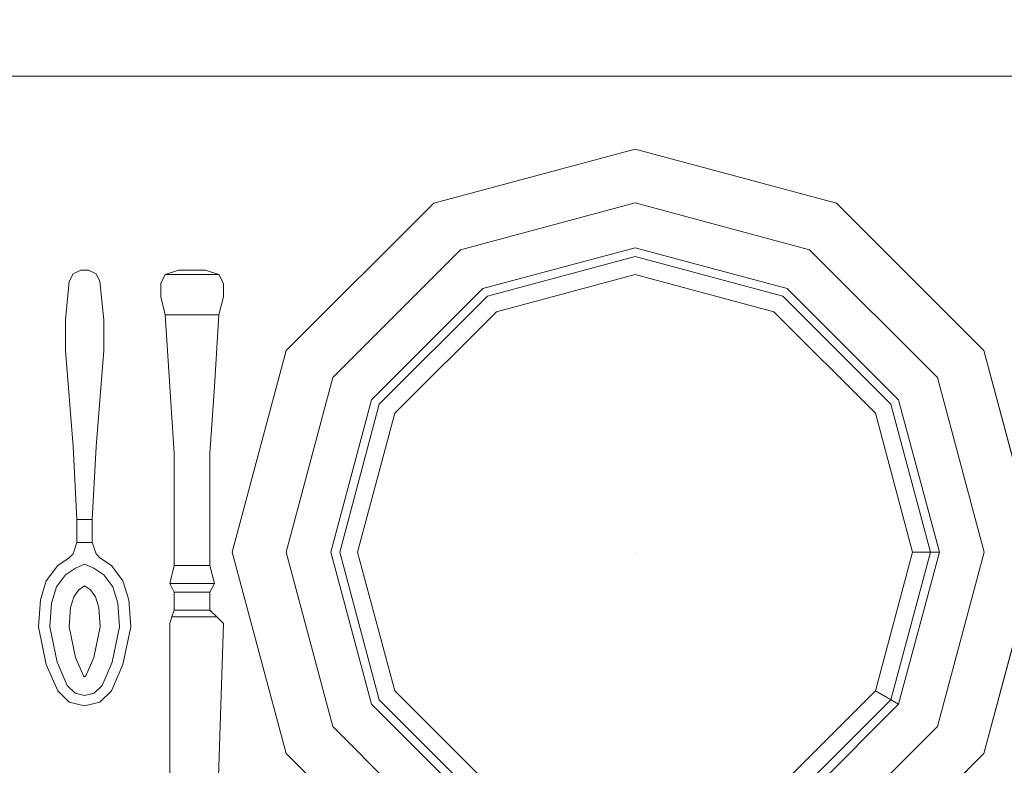
# Model space of a CAD drawing. Units: inches. Extents: x 375 to 1122, y 27 to 1069.
# Tile 135 of 155: x 717.62 to 731.16, y 906.27 to 916.52. Entities that reach past the tile are written whole.
import ezdxf

# ---------------------------------------------------------------- set-up
doc = ezdxf.new("R2010")
doc.units = ezdxf.units.IN
doc.layers.add('A-ANNO-DIMS', color=2, linetype='Continuous', lineweight=18)
doc.layers.add('Furniture', color=30, linetype='Continuous', lineweight=18)
doc.styles.get("Standard").update_dxf_attribs({"font": 'arial.ttf'})
doc.dimstyles.new('ISO-25', dxfattribs={"dimtxt": 12, "dimasz": 2.5, "dimexe": 1.5, "dimexo": 1.5, "dimtad": 1, "dimdec": 1, "dimlunit": 3, "dimtxsty": 'Standard', "dimblk": 'ARCHTICK', "dimcen": 2.5, "dimadec": 0, "dimazin": 0, "dimtfac": 1, "dimtdec": 1, "dimtmove": 0, "dimatfit": 3, "dimfxl": 1.5, "dimfxlon": 1, "dimarcsym": 0})

# ---------------------------------------------------------------- blocks, each defined once
blk = doc.blocks.new('A$C403C54AD')
blk.add_line((0.56427, 0.79569, -0.0006), (0.56427, 1.26108, -0.0006))
at = {"linetype": 'ByBlock'}
for points, invisible_edges in [([(0.72796, 1.16691, -0.0197), (0.72796, 1.14844, -0.0197), (0.66793, 1.13235, -0.0197), (0.6587, 1.14835, -0.0197)], 5), ([(0.72796, 1.13305, -0.03355), (0.72796, 1.16691, -0.02431), (0.6587, 1.14835, -0.02431), (0.67563, 1.11902, -0.03355)], 5), ([(0.79723, 1.14835, -0.0197), (0.78799, 1.13235, -0.0197), (0.72796, 1.14844, -0.0197), (0.72796, 1.16691, -0.0197)], 5), ([(0.7803, 1.11902, -0.03355), (0.79723, 1.14835, -0.02431), (0.72796, 1.16691, -0.02431), (0.72796, 1.13305, -0.03355)], 5), ([(0.6587, 1.14835, -0.0197), (0.66793, 1.13235, -0.0197), (0.62399, 1.08841, -0.0197), (0.60799, 1.09765, -0.0197)], 5), ([(0.67563, 1.11902, -0.03355), (0.6587, 1.14835, -0.02431), (0.60799, 1.09765, -0.02431), (0.63732, 1.08071, -0.03355)], 5), ([(0.72796, 1.14844, -0.0197), (0.72796, 1.12997, -0.02585), (0.67717, 1.11636, -0.02585), (0.66793, 1.13235, -0.0197)], 5), ([(0.78799, 1.13235, -0.0197), (0.77876, 1.11636, -0.02585), (0.72796, 1.12997, -0.02585), (0.72796, 1.14844, -0.0197)], 5), ([(0.81861, 1.08071, -0.03355), (0.84793, 1.09765, -0.02431), (0.79723, 1.14835, -0.02431), (0.7803, 1.11902, -0.03355)], 5), ([(0.84793, 1.09765, -0.0197), (0.83194, 1.08841, -0.0197), (0.78799, 1.13235, -0.0197), (0.79723, 1.14835, -0.0197)], 5), ([(0.66793, 1.13235, -0.0197), (0.67717, 1.11636, -0.02585), (0.63999, 1.07918, -0.02585), (0.62399, 1.08841, -0.0197)], 5), ([(0.72796, 1.12381, -0.04278), (0.72796, 1.13305, -0.03355), (0.67563, 1.11902, -0.03355), (0.68025, 1.11103, -0.04278)], 4), ([(0.83194, 1.08841, -0.0197), (0.81594, 1.07918, -0.02585), (0.77876, 1.11636, -0.02585), (0.78799, 1.13235, -0.0197)], 5), ([(0.72796, 1.12997, -0.02585), (0.72796, 1.02838, -0.02585), (0.72796, 1.02838, -0.02585), (0.67717, 1.11636, -0.02585)], 5), ([(0.77876, 1.11636, -0.02585), (0.72796, 1.02838, -0.02585), (0.72796, 1.02838, -0.02585), (0.72796, 1.12997, -0.02585)], 5), ([(0.68025, 1.11103, -0.04278), (0.67563, 1.11902, -0.03355), (0.63732, 1.08071, -0.03355), (0.64532, 1.0761, -0.04278)], 5), ([(0.81061, 1.0761, -0.04278), (0.81861, 1.08071, -0.03355), (0.7803, 1.11902, -0.03355), (0.77568, 1.11103, -0.04278)], 1), ([(0.67717, 1.11636, -0.02585), (0.72796, 1.02838, -0.02585), (0.72796, 1.02838, -0.02585), (0.63999, 1.07918, -0.02585)], 5), ([(0.81594, 1.07918, -0.02585), (0.72796, 1.02838, -0.02585), (0.72796, 1.02838, -0.02585), (0.77876, 1.11636, -0.02585)], 5), ([(0.60799, 1.09765, -0.0197), (0.62399, 1.08841, -0.0197), (0.60791, 1.02838, -0.0197), (0.58944, 1.02838, -0.0197)], 5), ([(0.63732, 1.08071, -0.03355), (0.60799, 1.09765, -0.02431), (0.58944, 1.02838, -0.02431), (0.6233, 1.02838, -0.03355)], 5), ([(0.62399, 1.08841, -0.0197), (0.63999, 1.07918, -0.02585), (0.62638, 1.02838, -0.02585), (0.60791, 1.02838, -0.0197)], 5), ([(0.64532, 1.0761, -0.04278), (0.63732, 1.08071, -0.03355), (0.6233, 1.02838, -0.03355), (0.63253, 1.02838, -0.04278)], 5), ([(0.63999, 1.07918, -0.02585), (0.72796, 1.02838, -0.02585), (0.72796, 1.02838, -0.02585), (0.62638, 1.02838, -0.02585)], 5), ([(0.82955, 1.02838, -0.02585), (0.72796, 1.02838, -0.02585), (0.72796, 1.02838, -0.02585), (0.81594, 1.07918, -0.02585)], 5), ([(0.58944, 1.02838, -0.0197), (0.60791, 1.02838, -0.0197), (0.62399, 0.96835, -0.0197), (0.60799, 0.95912, -0.0197)], 5), ([(0.6233, 1.02838, -0.03355), (0.58944, 1.02838, -0.02431), (0.60799, 0.95912, -0.02431), (0.63732, 0.97605, -0.03355)], 5), ([(0.60791, 1.02838, -0.0197), (0.62638, 1.02838, -0.02585), (0.63999, 0.97759, -0.02585), (0.62399, 0.96835, -0.0197)], 5), ([(0.63253, 1.02838, -0.04278), (0.6233, 1.02838, -0.03355), (0.63732, 0.97605, -0.03355), (0.64532, 0.98067, -0.04278)], 5), ([(0.62638, 1.02838, -0.02585), (0.72796, 1.02838, -0.02585), (0.72796, 1.02838, -0.02585), (0.63999, 0.97759, -0.02585)], 5), ([(0.63999, 0.97759, -0.02585), (0.72796, 1.02838, -0.02585), (0.72796, 1.02838, -0.02585), (0.67717, 0.94041, -0.02585)], 5), ([(0.67717, 0.94041, -0.02585), (0.72796, 1.02838, -0.02585), (0.72796, 1.02838, -0.02585), (0.72796, 0.9268, -0.02585)], 5), ([(0.81594, 0.97759, -0.02585), (0.72796, 1.02838, -0.02585), (0.72796, 1.02838, -0.02585), (0.82955, 1.02838, -0.02585)], 5), ([(0.77876, 0.94041, -0.02585), (0.72796, 1.02838, -0.02585), (0.72796, 1.02838, -0.02585), (0.81594, 0.97759, -0.02585)], 5), ([(0.72796, 0.9268, -0.02585), (0.72796, 1.02838, -0.02585), (0.72796, 1.02838, -0.02585), (0.77876, 0.94041, -0.02585)], 5), ([(0.64532, 0.98067, -0.04278), (0.63732, 0.97605, -0.03355), (0.67563, 0.93774, -0.03355), (0.68025, 0.94574, -0.04278)], 5), ([(0.77568, 0.94574, -0.04278), (0.7803, 0.93774, -0.03355), (0.81861, 0.97605, -0.03355), (0.81061, 0.98067, -0.04278)], 5), ([(0.63732, 0.97605, -0.03355), (0.60799, 0.95912, -0.02431), (0.6587, 0.90841, -0.02431), (0.67563, 0.93774, -0.03355)], 5), ([(0.62399, 0.96835, -0.0197), (0.63999, 0.97759, -0.02585), (0.67717, 0.94041, -0.02585), (0.66793, 0.92441, -0.0197)], 5), ([(0.78799, 0.92441, -0.0197), (0.77876, 0.94041, -0.02585), (0.81594, 0.97759, -0.02585), (0.83194, 0.96835, -0.0197)], 5), ([(0.7803, 0.93774, -0.03355), (0.79723, 0.90841, -0.02431), (0.84793, 0.95912, -0.02431), (0.81861, 0.97605, -0.03355)], 5), ([(0.60799, 0.95912, -0.0197), (0.62399, 0.96835, -0.0197), (0.66793, 0.92441, -0.0197), (0.6587, 0.90841, -0.0197)], 5), ([(0.79723, 0.90841, -0.0197), (0.78799, 0.92441, -0.0197), (0.83194, 0.96835, -0.0197), (0.84793, 0.95912, -0.0197)], 5), ([(0.68025, 0.94574, -0.04278), (0.67563, 0.93774, -0.03355), (0.72796, 0.92372, -0.03355), (0.72796, 0.93295, -0.04278)], 5), ([(0.72796, 0.93295, -0.04278), (0.72796, 0.92372, -0.03355), (0.7803, 0.93774, -0.03355), (0.77568, 0.94574, -0.04278)], 5), ([(0.66793, 0.92441, -0.0197), (0.67717, 0.94041, -0.02585), (0.72796, 0.9268, -0.02585), (0.72796, 0.90833, -0.0197)], 5), ([(0.72796, 0.90833, -0.0197), (0.72796, 0.9268, -0.02585), (0.77876, 0.94041, -0.02585), (0.78799, 0.92441, -0.0197)], 5), ([(0.67563, 0.93774, -0.03355), (0.6587, 0.90841, -0.02431), (0.72796, 0.88985, -0.02431), (0.72796, 0.92372, -0.03355)], 5), ([(0.72796, 0.92372, -0.03355), (0.72796, 0.88985, -0.02431), (0.79723, 0.90841, -0.02431), (0.7803, 0.93774, -0.03355)], 5), ([(0.6587, 0.90841, -0.0197), (0.66793, 0.92441, -0.0197), (0.72796, 0.90833, -0.0197), (0.72796, 0.88985, -0.0197)], 5), ([(0.72796, 0.88985, -0.0197), (0.72796, 0.90833, -0.0197), (0.78799, 0.92441, -0.0197), (0.79723, 0.90841, -0.0197)], 5)]:
    blk.add_3dface(points, dxfattribs=dict(at, invisible_edges=invisible_edges))
for points in [[(0.72796, 1.16691, -0.02431), (0.72796, 1.16691, -0.0197), (0.6587, 1.14835, -0.0197), (0.6587, 1.14835, -0.02431)], [(0.79723, 1.14835, -0.02431), (0.79723, 1.14835, -0.0197), (0.72796, 1.16691, -0.0197), (0.72796, 1.16691, -0.02431)], [(0.6587, 1.14835, -0.02431), (0.6587, 1.14835, -0.0197), (0.60799, 1.09765, -0.0197), (0.60799, 1.09765, -0.02431)], [(0.84793, 1.09765, -0.02431), (0.84793, 1.09765, -0.0197), (0.79723, 1.14835, -0.0197), (0.79723, 1.14835, -0.02431)], [(0.77568, 1.11103, -0.04278), (0.7803, 1.11902, -0.03355), (0.72796, 1.13305, -0.03355), (0.72796, 1.12381, -0.04278)], [(0.60799, 1.09765, -0.02431), (0.60799, 1.09765, -0.0197), (0.58944, 1.02838, -0.0197), (0.58944, 1.02838, -0.02431)], [(0.58944, 1.02838, -0.02431), (0.58944, 1.02838, -0.0197), (0.60799, 0.95912, -0.0197), (0.60799, 0.95912, -0.02431)], [(0.60799, 0.95912, -0.02431), (0.60799, 0.95912, -0.0197), (0.6587, 0.90841, -0.0197), (0.6587, 0.90841, -0.02431)], [(0.79723, 0.90841, -0.02431), (0.79723, 0.90841, -0.0197), (0.84793, 0.95912, -0.0197), (0.84793, 0.95912, -0.02431)], [(0.6587, 0.90841, -0.02431), (0.6587, 0.90841, -0.0197), (0.72796, 0.88985, -0.0197), (0.72796, 0.88985, -0.02431)], [(0.72796, 0.88985, -0.02431), (0.72796, 0.88985, -0.0197), (0.79723, 0.90841, -0.0197), (0.79723, 0.90841, -0.02431)]]:
    blk.add_3dface(points, dxfattribs=at)
for points in [[(0.63253, 0.88524, -0.03355), (0.63253, 0.86677, -0.03355), (0.63099, 0.87138, -0.03663), (0.63099, 0.88062, -0.03663)], [(0.63253, 0.88524, -0.03355), (0.63253, 0.88524, -0.03971), (0.63099, 0.88062, -0.03663)], [(0.63253, 0.88524, -0.03971), (0.63253, 0.86677, -0.03971), (0.63099, 0.87138, -0.03663), (0.63099, 0.88062, -0.03663)], [(0.63561, 0.88678, -0.04124), (0.63561, 0.88678, -0.03201), (0.63253, 0.88524, -0.03355), (0.63253, 0.88524, -0.03971)], [(0.64023, 0.88678, -0.03047), (0.64023, 0.88678, -0.04278), (0.63561, 0.88678, -0.04124), (0.63561, 0.88678, -0.03201)], [(0.64639, 0.88524, -0.04124), (0.64639, 0.88524, -0.03201), (0.64023, 0.88678, -0.03047), (0.64023, 0.88678, -0.04278)], [(0.67101, 0.8837, -0.03047), (0.67101, 0.8837, -0.04278), (0.64639, 0.88524, -0.04124), (0.64639, 0.88524, -0.03201)], [(0.75028, 0.88447, -0.03509), (0.75028, 0.86908, -0.03509), (0.74797, 0.86985, -0.03201), (0.74797, 0.88216, -0.03201)], [(0.75028, 0.88447, -0.03817), (0.75028, 0.86908, -0.03817), (0.74797, 0.86985, -0.04124), (0.74797, 0.88216, -0.04124)], [(0.6941, 0.88216, -0.04278), (0.6941, 0.88216, -0.03047), (0.67101, 0.8837, -0.03047), (0.67101, 0.8837, -0.04278)], [(0.73258, 0.88216, -0.03201), (0.73258, 0.88216, -0.04124), (0.6941, 0.88216, -0.04278), (0.6941, 0.88216, -0.03047)], [(0.73874, 0.86831, -0.03047), (0.73874, 0.8837, -0.03047), (0.73258, 0.88216, -0.03201), (0.73258, 0.86985, -0.03201)], [(0.73874, 0.86831, -0.04278), (0.73874, 0.8837, -0.04278), (0.73258, 0.88216, -0.04124), (0.73258, 0.86985, -0.04124)], [(0.73874, 0.8837, -0.04278), (0.73874, 0.8837, -0.03047), (0.73258, 0.88216, -0.03201), (0.73258, 0.88216, -0.04124)], [(0.74182, 0.88216, -0.03201), (0.74182, 0.86985, -0.03201), (0.73874, 0.86831, -0.03047), (0.73874, 0.8837, -0.03047)], [(0.74182, 0.88216, -0.04124), (0.74182, 0.86985, -0.04124), (0.73874, 0.86831, -0.04278), (0.73874, 0.8837, -0.04278)], [(0.74182, 0.88216, -0.03201), (0.74182, 0.88216, -0.04124), (0.73874, 0.8837, -0.04278), (0.73874, 0.8837, -0.03047)], [(0.74797, 0.86985, -0.03201), (0.74797, 0.88216, -0.03201), (0.74182, 0.88216, -0.03201), (0.74182, 0.86985, -0.03201)], [(0.74797, 0.86985, -0.04124), (0.74797, 0.88216, -0.04124), (0.74182, 0.88216, -0.04124), (0.74182, 0.86985, -0.04124)], [(0.63099, 0.87138, -0.03663), (0.63099, 0.87138, -0.03663), (0.63253, 0.86677, -0.03355), (0.63253, 0.86677, -0.03971)], [(0.64639, 0.86677, -0.03201), (0.64639, 0.86677, -0.04124), (0.67101, 0.86831, -0.04278), (0.67101, 0.86831, -0.03047)], [(0.67101, 0.86831, -0.04278), (0.67101, 0.86831, -0.03047), (0.6941, 0.86985, -0.03047), (0.6941, 0.86985, -0.04278)], [(0.6941, 0.86985, -0.03047), (0.6941, 0.86985, -0.04278), (0.73258, 0.86985, -0.04124), (0.73258, 0.86985, -0.03201)], [(0.73258, 0.86985, -0.04124), (0.73258, 0.86985, -0.03201), (0.73874, 0.86831, -0.03047), (0.73874, 0.86831, -0.04278)], [(0.73874, 0.86831, -0.03047), (0.73874, 0.86831, -0.04278), (0.74182, 0.86985, -0.04124), (0.74182, 0.86985, -0.03201)], [(0.63253, 0.86677, -0.03355), (0.63253, 0.86677, -0.03971), (0.63561, 0.86523, -0.04124), (0.63561, 0.86523, -0.03201)], [(0.63561, 0.86523, -0.03201), (0.63561, 0.86523, -0.04124), (0.64023, 0.86523, -0.04278), (0.64023, 0.86523, -0.03047)], [(0.64023, 0.86523, -0.04278), (0.64023, 0.86523, -0.03047), (0.64639, 0.86677, -0.03201), (0.64639, 0.86677, -0.04124)], [(0.74443, 0.85423, -0.03727), (0.74443, 0.85423, -0.03595), (0.73783, 0.85225, -0.03635), (0.73783, 0.85225, -0.03767)], [(0.75364, 0.85489, -0.0364), (0.75364, 0.85489, -0.03508), (0.74443, 0.85423, -0.03595), (0.74443, 0.85423, -0.03727)], [(0.76668, 0.85225, -0.03304), (0.76668, 0.85225, -0.03436), (0.75364, 0.85489, -0.0364), (0.75364, 0.85489, -0.03508)], [(0.73783, 0.85225, -0.03635), (0.73783, 0.85225, -0.03767), (0.73257, 0.8483, -0.03815), (0.73257, 0.8483, -0.03683)], [(0.77574, 0.8483, -0.03252), (0.77574, 0.8483, -0.03121), (0.76668, 0.85225, -0.03304), (0.76668, 0.85225, -0.03436)], [(0.73257, 0.8483, -0.03815), (0.73257, 0.8483, -0.03683), (0.72996, 0.84434, -0.03721), (0.72996, 0.84434, -0.03936)], [(0.77958, 0.84434, -0.03012), (0.77958, 0.84434, -0.03144), (0.77574, 0.8483, -0.03252), (0.77574, 0.8483, -0.03121)], [(0.63495, 0.84434, -0.03878), (0.63495, 0.84434, -0.04275), (0.63231, 0.84302, -0.04254), (0.63231, 0.84302, -0.03857)], [(0.64814, 0.84566, -0.04278), (0.64814, 0.84566, -0.03881), (0.63495, 0.84434, -0.03878), (0.63495, 0.84434, -0.04275)], [(0.6587, 0.84566, -0.03853), (0.6587, 0.84566, -0.0425), (0.64814, 0.84566, -0.04278), (0.64814, 0.84566, -0.03881)], [(0.78089, 0.83906, -0.03125), (0.78089, 0.83906, -0.02993), (0.77958, 0.84434, -0.03012), (0.77958, 0.84434, -0.03144)], [(0.63231, 0.84302, -0.04254), (0.63231, 0.84302, -0.03857), (0.63099, 0.84038, -0.03871), (0.63099, 0.84038, -0.04225)], [(0.63099, 0.84038, -0.03871), (0.63099, 0.84038, -0.04225), (0.63099, 0.83774, -0.04225), (0.63099, 0.83774, -0.03871)], [(0.71675, 0.8417, -0.03621), (0.71675, 0.83642, -0.03621), (0.72466, 0.83642, -0.03684), (0.72466, 0.8417, -0.03684)], [(0.71675, 0.8417, -0.03399), (0.71675, 0.83642, -0.03399), (0.72466, 0.83642, -0.03462), (0.72466, 0.8417, -0.03462)], [(0.63099, 0.83774, -0.04225), (0.63099, 0.83774, -0.03871), (0.63231, 0.8351, -0.03857), (0.63231, 0.8351, -0.04254)], [(0.77958, 0.83378, -0.03012), (0.77958, 0.83378, -0.03144), (0.78089, 0.83906, -0.03125), (0.78089, 0.83906, -0.02993)], [(0.63231, 0.8351, -0.03857), (0.63231, 0.8351, -0.04254), (0.63495, 0.83378, -0.04275), (0.63495, 0.83378, -0.03878)], [(0.63495, 0.83378, -0.04275), (0.63495, 0.83378, -0.03878), (0.64814, 0.83247, -0.03881), (0.64814, 0.83247, -0.04278)], [(0.72996, 0.83378, -0.03936), (0.72996, 0.83378, -0.03721), (0.73257, 0.82983, -0.03683), (0.73257, 0.82983, -0.03815)], [(0.77574, 0.82983, -0.03252), (0.77574, 0.82983, -0.03121), (0.77958, 0.83378, -0.03012), (0.77958, 0.83378, -0.03144)], [(0.64814, 0.83247, -0.03881), (0.64814, 0.83247, -0.04278), (0.6587, 0.83247, -0.0425), (0.6587, 0.83247, -0.03853)], [(0.73257, 0.82983, -0.03683), (0.73257, 0.82983, -0.03815), (0.73783, 0.82587, -0.03767), (0.73783, 0.82587, -0.03635)], [(0.76668, 0.82587, -0.03304), (0.76668, 0.82587, -0.03436), (0.77574, 0.82983, -0.03252), (0.77574, 0.82983, -0.03121)], [(0.73783, 0.82587, -0.03767), (0.73783, 0.82587, -0.03635), (0.74443, 0.82389, -0.03595), (0.74443, 0.82389, -0.03727)], [(0.74443, 0.82389, -0.03595), (0.74443, 0.82389, -0.03727), (0.75364, 0.82323, -0.0364), (0.75364, 0.82323, -0.03508)], [(0.75364, 0.82323, -0.0364), (0.75364, 0.82323, -0.03508), (0.76668, 0.82587, -0.03304), (0.76668, 0.82587, -0.03436)]]:
    blk.add_3dface(points)
for points, invisible_edges in [([(0.63561, 0.86523, -0.03201), (0.63561, 0.88678, -0.03201), (0.63253, 0.88524, -0.03355), (0.63253, 0.86677, -0.03355)], 1), ([(0.63561, 0.86523, -0.04124), (0.63561, 0.88678, -0.04124), (0.63253, 0.88524, -0.03971), (0.63253, 0.86677, -0.03971)], 1), ([(0.64023, 0.88678, -0.03047), (0.64023, 0.86523, -0.03047), (0.63561, 0.86523, -0.03201), (0.63561, 0.88678, -0.03201)], 5), ([(0.64023, 0.88678, -0.04278), (0.64023, 0.86523, -0.04278), (0.63561, 0.86523, -0.04124), (0.63561, 0.88678, -0.04124)], 5), ([(0.64639, 0.86677, -0.03201), (0.64639, 0.88524, -0.03201), (0.64023, 0.88678, -0.03047), (0.64023, 0.86523, -0.03047)], 4), ([(0.64639, 0.86677, -0.04124), (0.64639, 0.88524, -0.04124), (0.64023, 0.88678, -0.04278), (0.64023, 0.86523, -0.04278)], 4), ([(0.67101, 0.8837, -0.03047), (0.67101, 0.86831, -0.03047), (0.64639, 0.86677, -0.03201), (0.64639, 0.88524, -0.03201)], 1), ([(0.67101, 0.8837, -0.04278), (0.67101, 0.86831, -0.04278), (0.64639, 0.86677, -0.04124), (0.64639, 0.88524, -0.04124)], 1), ([(0.75028, 0.88447, -0.03509), (0.75028, 0.88447, -0.03817), (0.74797, 0.88216, -0.04124), (0.74797, 0.88216, -0.03201)], 5), ([(0.75259, 0.88678, -0.03586), (0.75259, 0.86831, -0.03586), (0.75028, 0.86908, -0.03509), (0.75028, 0.88447, -0.03509)], 1), ([(0.75259, 0.88678, -0.0374), (0.75259, 0.86831, -0.0374), (0.75028, 0.86908, -0.03817), (0.75028, 0.88447, -0.03817)], 1), ([(0.75259, 0.88678, -0.0374), (0.75259, 0.88678, -0.03586), (0.75028, 0.88447, -0.03509), (0.75028, 0.88447, -0.03817)], 5), ([(0.81108, 0.86831, -0.03586), (0.84956, 0.8837, -0.03586), (0.75259, 0.88678, -0.03586), (0.75259, 0.86831, -0.03586)], 5), ([(0.81108, 0.86831, -0.0374), (0.84956, 0.8837, -0.0374), (0.75259, 0.88678, -0.0374), (0.75259, 0.86831, -0.0374)], 5), ([(0.84956, 0.8837, -0.0374), (0.84956, 0.8837, -0.03586), (0.75259, 0.88678, -0.03586), (0.75259, 0.88678, -0.0374)], 5), ([(0.6941, 0.86985, -0.03047), (0.6941, 0.88216, -0.03047), (0.67101, 0.8837, -0.03047), (0.67101, 0.86831, -0.03047)], 5), ([(0.6941, 0.86985, -0.04278), (0.6941, 0.88216, -0.04278), (0.67101, 0.8837, -0.04278), (0.67101, 0.86831, -0.04278)], 5), ([(0.73258, 0.88216, -0.03201), (0.73258, 0.86985, -0.03201), (0.6941, 0.86985, -0.03047), (0.6941, 0.88216, -0.03047)], 4), ([(0.73258, 0.88216, -0.04124), (0.73258, 0.86985, -0.04124), (0.6941, 0.86985, -0.04278), (0.6941, 0.88216, -0.04278)], 4), ([(0.74797, 0.88216, -0.04124), (0.74797, 0.88216, -0.03201), (0.74182, 0.88216, -0.03201), (0.74182, 0.88216, -0.04124)], 1), ([(0.74182, 0.86985, -0.04124), (0.74182, 0.86985, -0.03201), (0.74797, 0.86985, -0.03201), (0.74797, 0.86985, -0.04124)], 4), ([(0.74797, 0.86985, -0.03201), (0.74797, 0.86985, -0.04124), (0.75028, 0.86908, -0.03817), (0.75028, 0.86908, -0.03509)], 5), ([(0.75028, 0.86908, -0.03817), (0.75028, 0.86908, -0.03509), (0.75259, 0.86831, -0.03586), (0.75259, 0.86831, -0.0374)], 5), ([(0.75259, 0.86831, -0.03586), (0.75259, 0.86831, -0.0374), (0.81108, 0.86831, -0.0374), (0.81108, 0.86831, -0.03586)], 5), ([(0.73998, 0.84876, -0.03894), (0.73783, 0.85225, -0.03635), (0.74443, 0.85423, -0.03595), (0.7455, 0.85042, -0.03843)], 5), ([(0.73998, 0.84876, -0.04026), (0.73783, 0.85225, -0.03767), (0.74443, 0.85423, -0.03727), (0.7455, 0.85042, -0.03975)], 5), ([(0.74443, 0.85423, -0.03595), (0.7455, 0.85042, -0.03843), (0.75374, 0.85101, -0.03754), (0.75364, 0.85489, -0.03508)], 5), ([(0.74443, 0.85423, -0.03727), (0.7455, 0.85042, -0.03975), (0.75374, 0.85101, -0.03886), (0.75364, 0.85489, -0.0364)], 5), ([(0.75374, 0.85101, -0.03886), (0.75364, 0.85489, -0.0364), (0.76668, 0.85225, -0.03436), (0.76587, 0.84855, -0.03687)], 5), ([(0.75374, 0.85101, -0.03754), (0.75364, 0.85489, -0.03508), (0.76668, 0.85225, -0.03304), (0.76587, 0.84855, -0.03555)], 5), ([(0.73257, 0.8483, -0.03815), (0.73576, 0.84561, -0.04043), (0.73998, 0.84876, -0.04026), (0.73783, 0.85225, -0.03767)], 5), ([(0.73257, 0.8483, -0.03683), (0.73576, 0.84561, -0.03911), (0.73998, 0.84876, -0.03894), (0.73783, 0.85225, -0.03635)], 5), ([(0.74707, 0.84391, -0.04103), (0.7455, 0.85042, -0.03843), (0.73998, 0.84876, -0.03894), (0.74335, 0.84279, -0.04126)], 5), ([(0.75374, 0.85101, -0.03886), (0.75368, 0.84439, -0.0414), (0.74707, 0.84391, -0.04234), (0.7455, 0.85042, -0.03975)], 5), ([(0.75374, 0.85101, -0.03754), (0.75368, 0.84439, -0.04008), (0.74707, 0.84391, -0.04103), (0.7455, 0.85042, -0.03843)], 5), ([(0.76429, 0.84224, -0.03837), (0.76587, 0.84855, -0.03555), (0.75374, 0.85101, -0.03754), (0.75368, 0.84439, -0.04008)], 5), ([(0.76429, 0.84224, -0.03969), (0.76587, 0.84855, -0.03687), (0.75374, 0.85101, -0.03886), (0.75368, 0.84439, -0.0414)], 5), ([(0.76668, 0.85225, -0.03436), (0.76587, 0.84855, -0.03687), (0.7739, 0.84505, -0.03516), (0.77574, 0.8483, -0.03252)], 5), ([(0.76668, 0.85225, -0.03304), (0.76587, 0.84855, -0.03555), (0.7739, 0.84505, -0.03385), (0.77574, 0.8483, -0.03121)], 5), ([(0.73347, 0.8422, -0.03912), (0.72996, 0.84434, -0.03721), (0.73257, 0.8483, -0.03683), (0.73576, 0.84561, -0.03911)], 5), ([(0.73998, 0.84876, -0.04026), (0.74335, 0.84279, -0.04258), (0.74098, 0.84102, -0.04267), (0.73576, 0.84561, -0.04043)], 5), ([(0.73998, 0.84876, -0.03894), (0.74335, 0.84279, -0.04126), (0.74098, 0.84102, -0.04136), (0.73576, 0.84561, -0.03911)], 5), ([(0.7739, 0.84505, -0.03516), (0.77052, 0.8395, -0.03806), (0.76429, 0.84224, -0.03969), (0.76587, 0.84855, -0.03687)], 5), ([(0.7739, 0.84505, -0.03385), (0.77052, 0.8395, -0.03674), (0.76429, 0.84224, -0.03837), (0.76587, 0.84855, -0.03555)], 5), ([(0.7739, 0.84505, -0.03516), (0.77574, 0.8483, -0.03252), (0.77958, 0.84434, -0.03144), (0.77652, 0.84237, -0.03461)], 5), ([(0.7739, 0.84505, -0.03385), (0.77574, 0.8483, -0.03121), (0.77958, 0.84434, -0.03012), (0.77652, 0.84237, -0.03329)], 5), ([(0.63231, 0.8351, -0.03857), (0.63231, 0.84302, -0.03857), (0.63495, 0.84434, -0.03878), (0.63495, 0.83378, -0.03878)], 5), ([(0.63231, 0.8351, -0.04254), (0.63231, 0.84302, -0.04254), (0.63495, 0.84434, -0.04275), (0.63495, 0.83378, -0.04275)], 5), ([(0.63495, 0.84434, -0.03878), (0.63495, 0.83378, -0.03878), (0.64814, 0.83247, -0.03881), (0.64814, 0.84566, -0.03881)], 5), ([(0.63495, 0.84434, -0.04275), (0.63495, 0.83378, -0.04275), (0.64814, 0.83247, -0.04278), (0.64814, 0.84566, -0.04278)], 5), ([(0.64814, 0.83247, -0.03881), (0.64814, 0.84566, -0.03881), (0.6587, 0.84566, -0.03853), (0.6587, 0.83247, -0.03853)], 5), ([(0.64814, 0.83247, -0.04278), (0.64814, 0.84566, -0.04278), (0.6587, 0.84566, -0.0425), (0.6587, 0.83247, -0.0425)], 5), ([(0.6587, 0.84566, -0.0425), (0.6587, 0.83247, -0.0425), (0.69168, 0.8351, -0.03912), (0.69168, 0.84302, -0.03912)], 5), ([(0.69168, 0.84302, -0.03912), (0.69168, 0.84302, -0.03648), (0.6587, 0.84566, -0.03853), (0.6587, 0.84566, -0.0425)], 1), ([(0.6587, 0.84566, -0.03853), (0.6587, 0.83247, -0.03853), (0.69168, 0.8351, -0.03648), (0.69168, 0.84302, -0.03648)], 5), ([(0.72862, 0.84302, -0.03647), (0.72862, 0.8351, -0.03647), (0.72996, 0.83378, -0.03721), (0.72996, 0.84434, -0.03721)], 5), ([(0.72862, 0.84302, -0.03856), (0.72862, 0.8351, -0.03856), (0.72996, 0.83378, -0.03936), (0.72996, 0.84434, -0.03936)], 5), ([(0.72862, 0.84302, -0.03647), (0.72862, 0.84302, -0.03856), (0.72996, 0.84434, -0.03936), (0.72996, 0.84434, -0.03721)], 1), ([(0.72996, 0.84434, -0.03936), (0.72996, 0.83906, -0.03936), (0.73211, 0.83906, -0.04026), (0.73347, 0.8422, -0.04044)], 11), ([(0.72996, 0.84434, -0.03721), (0.72996, 0.83906, -0.03721), (0.73211, 0.83906, -0.03894), (0.73347, 0.8422, -0.03912)], 11), ([(0.74098, 0.84102, -0.04267), (0.73576, 0.84561, -0.04043), (0.73347, 0.8422, -0.04044), (0.73963, 0.83906, -0.04247)], 5), ([(0.74098, 0.84102, -0.04136), (0.73576, 0.84561, -0.03911), (0.73347, 0.8422, -0.03912), (0.73963, 0.83906, -0.04116)], 5), ([(0.74707, 0.83421, -0.04234), (0.74707, 0.84391, -0.04234), (0.74335, 0.84279, -0.04258), (0.74335, 0.83533, -0.04258)], 5), ([(0.74707, 0.83421, -0.04103), (0.74707, 0.84391, -0.04103), (0.74335, 0.84279, -0.04126), (0.74335, 0.83533, -0.04126)], 5), ([(0.75368, 0.84439, -0.0414), (0.75368, 0.83374, -0.0414), (0.74707, 0.83421, -0.04234), (0.74707, 0.84391, -0.04234)], 5), ([(0.75368, 0.84439, -0.04008), (0.75368, 0.83374, -0.04008), (0.74707, 0.83421, -0.04103), (0.74707, 0.84391, -0.04103)], 5), ([(0.76429, 0.83589, -0.03837), (0.76429, 0.84224, -0.03837), (0.75368, 0.84439, -0.04008), (0.75368, 0.83374, -0.04008)], 5), ([(0.76429, 0.83589, -0.03969), (0.76429, 0.84224, -0.03969), (0.75368, 0.84439, -0.0414), (0.75368, 0.83374, -0.0414)], 5), ([(0.77052, 0.8395, -0.03674), (0.77652, 0.84237, -0.03329), (0.7739, 0.84505, -0.03385), (0.77052, 0.8395, -0.03674)], 5), ([(0.77052, 0.8395, -0.03806), (0.77652, 0.84237, -0.03461), (0.7739, 0.84505, -0.03516), (0.77052, 0.8395, -0.03806)], 5), ([(0.77958, 0.84434, -0.03144), (0.77652, 0.84237, -0.03461), (0.77733, 0.83906, -0.03442), (0.78089, 0.83906, -0.03125)], 5), ([(0.77958, 0.84434, -0.03012), (0.77652, 0.84237, -0.03329), (0.77733, 0.83906, -0.0331), (0.78089, 0.83906, -0.02993)], 5), ([(0.63099, 0.84038, -0.03871), (0.63099, 0.83774, -0.03871), (0.63231, 0.8351, -0.03857), (0.63231, 0.84302, -0.03857)], 4), ([(0.63099, 0.84038, -0.04225), (0.63099, 0.83774, -0.04225), (0.63231, 0.8351, -0.04254), (0.63231, 0.84302, -0.04254)], 4), ([(0.69168, 0.8351, -0.03648), (0.69168, 0.84302, -0.03648), (0.71675, 0.8417, -0.03399), (0.71675, 0.83642, -0.03399)], 1), ([(0.71675, 0.8417, -0.03399), (0.71675, 0.8417, -0.03621), (0.69168, 0.84302, -0.03912), (0.69168, 0.84302, -0.03648)], 5), ([(0.69168, 0.8351, -0.03912), (0.69168, 0.84302, -0.03912), (0.71675, 0.8417, -0.03621), (0.71675, 0.83642, -0.03621)], 1), ([(0.72466, 0.8417, -0.03684), (0.72466, 0.8417, -0.03462), (0.71675, 0.8417, -0.03399), (0.71675, 0.8417, -0.03621)], 5), ([(0.72466, 0.83642, -0.03462), (0.72466, 0.8417, -0.03462), (0.72862, 0.84302, -0.03647), (0.72862, 0.8351, -0.03647)], 4), ([(0.72466, 0.8417, -0.03684), (0.72466, 0.8417, -0.03462), (0.72862, 0.84302, -0.03647), (0.72862, 0.84302, -0.03856)], 5), ([(0.72466, 0.83642, -0.03684), (0.72466, 0.8417, -0.03684), (0.72862, 0.84302, -0.03856), (0.72862, 0.8351, -0.03856)], 4), ([(0.73347, 0.8422, -0.04044), (0.73963, 0.83906, -0.04247), (0.73963, 0.83906, -0.04247), (0.73211, 0.83906, -0.04026)], 5), ([(0.73347, 0.8422, -0.03912), (0.73963, 0.83906, -0.04116), (0.73963, 0.83906, -0.04116), (0.73211, 0.83906, -0.03894)], 5), ([(0.74098, 0.8371, -0.04267), (0.74098, 0.84102, -0.04267), (0.73963, 0.83906, -0.04247)], 1), ([(0.74098, 0.8371, -0.04136), (0.74098, 0.84102, -0.04136), (0.73963, 0.83906, -0.04116)], 1), ([(0.74335, 0.84279, -0.04258), (0.74335, 0.83533, -0.04258), (0.74098, 0.8371, -0.04267), (0.74098, 0.84102, -0.04267)], 5), ([(0.74335, 0.84279, -0.04126), (0.74335, 0.83533, -0.04126), (0.74098, 0.8371, -0.04136), (0.74098, 0.84102, -0.04136)], 5), ([(0.77052, 0.8395, -0.03806), (0.77052, 0.83862, -0.03806), (0.76429, 0.83589, -0.03969), (0.76429, 0.84224, -0.03969)], 5), ([(0.77052, 0.8395, -0.03674), (0.77052, 0.83862, -0.03674), (0.76429, 0.83589, -0.03837), (0.76429, 0.84224, -0.03837)], 5), ([(0.77733, 0.83906, -0.0331), (0.77094, 0.83906, -0.0366), (0.77052, 0.8395, -0.03674), (0.77652, 0.84237, -0.03329)], 5), ([(0.77733, 0.83906, -0.03442), (0.77094, 0.83906, -0.03792), (0.77052, 0.8395, -0.03806), (0.77652, 0.84237, -0.03461)], 5), ([(0.72996, 0.83378, -0.03936), (0.72996, 0.83906, -0.03936), (0.73211, 0.83906, -0.04026), (0.73347, 0.83592, -0.04044)], 11), ([(0.72996, 0.83378, -0.03721), (0.72996, 0.83906, -0.03721), (0.73211, 0.83906, -0.03894), (0.73347, 0.83592, -0.03912)], 11), ([(0.73347, 0.83592, -0.04044), (0.73963, 0.83906, -0.04247), (0.73963, 0.83906, -0.04247), (0.73211, 0.83906, -0.04026)], 5), ([(0.73347, 0.83592, -0.03912), (0.73963, 0.83906, -0.04116), (0.73963, 0.83906, -0.04116), (0.73211, 0.83906, -0.03894)], 5), ([(0.74098, 0.8371, -0.04267), (0.73576, 0.83251, -0.04043), (0.73347, 0.83592, -0.04044), (0.73963, 0.83906, -0.04247)], 5), ([(0.74098, 0.8371, -0.04136), (0.73576, 0.83251, -0.03911), (0.73347, 0.83592, -0.03912), (0.73963, 0.83906, -0.04116)], 5), ([(0.73998, 0.82936, -0.04026), (0.74335, 0.83533, -0.04258), (0.74098, 0.8371, -0.04267), (0.73576, 0.83251, -0.04043)], 5), ([(0.73998, 0.82936, -0.03894), (0.74335, 0.83533, -0.04126), (0.74098, 0.8371, -0.04136), (0.73576, 0.83251, -0.03911)], 5), ([(0.7739, 0.83308, -0.03516), (0.77052, 0.83862, -0.03806), (0.76429, 0.83589, -0.03969), (0.76587, 0.82957, -0.03687)], 5), ([(0.7739, 0.83308, -0.03385), (0.77052, 0.83862, -0.03674), (0.76429, 0.83589, -0.03837), (0.76587, 0.82957, -0.03555)], 5), ([(0.77094, 0.83906, -0.0366), (0.77052, 0.83862, -0.03674), (0.77052, 0.8395, -0.03674), (0.77094, 0.83906, -0.0366)], 2), ([(0.77094, 0.83906, -0.03792), (0.77052, 0.83862, -0.03806), (0.77052, 0.8395, -0.03806), (0.77094, 0.83906, -0.03792)], 2), ([(0.77733, 0.83906, -0.0331), (0.77094, 0.83906, -0.0366), (0.77052, 0.83862, -0.03674), (0.77652, 0.83575, -0.03329)], 5), ([(0.77733, 0.83906, -0.03442), (0.77094, 0.83906, -0.03792), (0.77052, 0.83862, -0.03806), (0.77652, 0.83575, -0.03461)], 5), ([(0.77052, 0.83862, -0.03674), (0.77652, 0.83575, -0.03329), (0.7739, 0.83308, -0.03385), (0.77052, 0.83862, -0.03674)], 5), ([(0.77052, 0.83862, -0.03806), (0.77652, 0.83575, -0.03461), (0.7739, 0.83308, -0.03516), (0.77052, 0.83862, -0.03806)], 5), ([(0.77958, 0.83378, -0.03144), (0.77652, 0.83575, -0.03461), (0.77733, 0.83906, -0.03442), (0.78089, 0.83906, -0.03125)], 5), ([(0.77958, 0.83378, -0.03012), (0.77652, 0.83575, -0.03329), (0.77733, 0.83906, -0.0331), (0.78089, 0.83906, -0.02993)], 5), ([(0.6587, 0.83247, -0.0425), (0.6587, 0.83247, -0.03853), (0.69168, 0.8351, -0.03648), (0.69168, 0.8351, -0.03912)], 4), ([(0.69168, 0.8351, -0.03648), (0.69168, 0.8351, -0.03912), (0.71675, 0.83642, -0.03621), (0.71675, 0.83642, -0.03399)], 5), ([(0.71675, 0.83642, -0.03621), (0.71675, 0.83642, -0.03399), (0.72466, 0.83642, -0.03462), (0.72466, 0.83642, -0.03684)], 5), ([(0.72466, 0.83642, -0.03462), (0.72466, 0.83642, -0.03684), (0.72862, 0.8351, -0.03856), (0.72862, 0.8351, -0.03647)], 5), ([(0.72862, 0.8351, -0.03856), (0.72862, 0.8351, -0.03647), (0.72996, 0.83378, -0.03721), (0.72996, 0.83378, -0.03936)], 1), ([(0.73347, 0.83592, -0.04044), (0.72996, 0.83378, -0.03936), (0.73257, 0.82983, -0.03815), (0.73576, 0.83251, -0.04043)], 5), ([(0.73347, 0.83592, -0.03912), (0.72996, 0.83378, -0.03721), (0.73257, 0.82983, -0.03683), (0.73576, 0.83251, -0.03911)], 5), ([(0.74707, 0.83421, -0.04234), (0.7455, 0.8277, -0.03975), (0.73998, 0.82936, -0.04026), (0.74335, 0.83533, -0.04258)], 5), ([(0.74707, 0.83421, -0.04103), (0.7455, 0.8277, -0.03843), (0.73998, 0.82936, -0.03894), (0.74335, 0.83533, -0.04126)], 5), ([(0.75374, 0.82711, -0.03886), (0.75368, 0.83374, -0.0414), (0.74707, 0.83421, -0.04234), (0.7455, 0.8277, -0.03975)], 5), ([(0.75374, 0.82711, -0.03754), (0.75368, 0.83374, -0.04008), (0.74707, 0.83421, -0.04103), (0.7455, 0.8277, -0.03843)], 5), ([(0.76429, 0.83589, -0.03837), (0.76587, 0.82957, -0.03555), (0.75374, 0.82711, -0.03754), (0.75368, 0.83374, -0.04008)], 5), ([(0.76429, 0.83589, -0.03969), (0.76587, 0.82957, -0.03687), (0.75374, 0.82711, -0.03886), (0.75368, 0.83374, -0.0414)], 5), ([(0.76668, 0.82587, -0.03436), (0.76587, 0.82957, -0.03687), (0.7739, 0.83308, -0.03516), (0.77574, 0.82983, -0.03252)], 5), ([(0.76668, 0.82587, -0.03304), (0.76587, 0.82957, -0.03555), (0.7739, 0.83308, -0.03385), (0.77574, 0.82983, -0.03121)], 5), ([(0.7739, 0.83308, -0.03516), (0.77574, 0.82983, -0.03252), (0.77958, 0.83378, -0.03144), (0.77652, 0.83575, -0.03461)], 5), ([(0.7739, 0.83308, -0.03385), (0.77574, 0.82983, -0.03121), (0.77958, 0.83378, -0.03012), (0.77652, 0.83575, -0.03329)], 5), ([(0.73257, 0.82983, -0.03815), (0.73576, 0.83251, -0.04043), (0.73998, 0.82936, -0.04026), (0.73783, 0.82587, -0.03767)], 5), ([(0.73257, 0.82983, -0.03683), (0.73576, 0.83251, -0.03911), (0.73998, 0.82936, -0.03894), (0.73783, 0.82587, -0.03635)], 5), ([(0.73998, 0.82936, -0.03894), (0.73783, 0.82587, -0.03635), (0.74443, 0.82389, -0.03595), (0.7455, 0.8277, -0.03843)], 5), ([(0.73998, 0.82936, -0.04026), (0.73783, 0.82587, -0.03767), (0.74443, 0.82389, -0.03727), (0.7455, 0.8277, -0.03975)], 5), ([(0.74443, 0.82389, -0.03595), (0.7455, 0.8277, -0.03843), (0.75374, 0.82711, -0.03754), (0.75364, 0.82323, -0.03508)], 5), ([(0.74443, 0.82389, -0.03727), (0.7455, 0.8277, -0.03975), (0.75374, 0.82711, -0.03886), (0.75364, 0.82323, -0.0364)], 5), ([(0.75374, 0.82711, -0.03886), (0.75364, 0.82323, -0.0364), (0.76668, 0.82587, -0.03436), (0.76587, 0.82957, -0.03687)], 5), ([(0.75374, 0.82711, -0.03754), (0.75364, 0.82323, -0.03508), (0.76668, 0.82587, -0.03304), (0.76587, 0.82957, -0.03555)], 5)]:
    blk.add_3dface(points, dxfattribs=dict(invisible_edges=invisible_edges))
blk = doc.blocks.new('_ArchTick')
at = {"color": 0, "linetype": 'ByBlock', "const_width": 0.15}
blk.add_lwpolyline([(-0.5, -0.5), (0.5, 0.5)], dxfattribs=at)
blk = doc.blocks.new('*D73')
at = {"layer": 'A-ANNO-DIMS', "color": 0, "lineweight": -2, "transparency": 16777216}
for p, q in [((686.757, 932.428), (686.757, 929.428)), ((770.757, 932.428), (770.757, 929.428)), ((686.757, 930.928), (770.757, 930.928)), ((770.757, 930.928), (987.61, 930.928))]:
    blk.add_line(p, q, dxfattribs=at)
at = {"layer": 'Defpoints', "color": 0, "transparency": 16777216}
for p in [(686.757, 943.528), (770.757, 943.528), (770.757, 930.928)]:
    blk.add_point(p, dxfattribs=at)
at = {"layer": 'A-ANNO-DIMS', "color": 0, "lineweight": -2, "transparency": 16777216, "xscale": 2.5, "yscale": 2.5, "zscale": 2.5, "rotation": 180}
blk.add_blockref('_ArchTick', (686.757, 930.928), dxfattribs=at)
at = {"layer": 'A-ANNO-DIMS', "color": 0, "lineweight": -2, "transparency": 16777216, "xscale": 2.5, "yscale": 2.5, "zscale": 2.5}
blk.add_blockref('_ArchTick', (770.757, 930.928), dxfattribs=at)
at = {"layer": 'A-ANNO-DIMS', "color": 0, "transparency": 16777216, "insert": (880.433, 937.757), "char_height": 12, "attachment_point": 5}
blk.add_mtext('2-PANEL SLIDER 7\'-0" TYP.', dxfattribs=at)
blk = doc.blocks.new('*D88')
at = {"layer": 'A-ANNO-DIMS', "color": 0, "lineweight": -2, "transparency": 16777216}
for p, q in [((731.007, 1052.528), (731.007, 1055.528)), ((854.007, 1052.528), (854.007, 1055.528)), ((731.007, 1054.028), (854.007, 1054.028))]:
    blk.add_line(p, q, dxfattribs=at)
at = {"layer": 'Defpoints', "color": 0, "transparency": 16777216}
for p in [(854.007, 1054.028), (731.007, 502.528), (854.007, 502.528)]:
    blk.add_point(p, dxfattribs=at)
at = {"layer": 'A-ANNO-DIMS', "color": 0, "lineweight": -2, "transparency": 16777216, "xscale": 2.5, "yscale": 2.5, "zscale": 2.5, "rotation": 180}
blk.add_blockref('_ArchTick', (731.007, 1054.028), dxfattribs=at)
at = {"layer": 'A-ANNO-DIMS', "color": 0, "lineweight": -2, "transparency": 16777216, "xscale": 2.5, "yscale": 2.5, "zscale": 2.5}
blk.add_blockref('_ArchTick', (854.007, 1054.028), dxfattribs=at)
at = {"layer": 'A-ANNO-DIMS', "color": 0, "transparency": 16777216, "insert": (792.507, 1060.784), "char_height": 12, "attachment_point": 5}
blk.add_mtext('10\'-3"', dxfattribs=at)
blk = doc.blocks.new('*D91')
at = {"layer": 'A-ANNO-DIMS', "color": 0, "lineweight": -2, "transparency": 16777216}
for p, q in [((728.007, 1052.528), (728.007, 1055.528)), ((788.007, 1052.528), (788.007, 1055.528)), ((728.007, 1054.028), (788.007, 1054.028))]:
    blk.add_line(p, q, dxfattribs=at)
at = {"layer": 'Defpoints', "color": 0, "transparency": 16777216}
for p in [(788.007, 1054.028), (728.007, 774.028), (788.007, 774.028)]:
    blk.add_point(p, dxfattribs=at)
at = {"layer": 'A-ANNO-DIMS', "color": 0, "lineweight": -2, "transparency": 16777216, "xscale": 2.5, "yscale": 2.5, "zscale": 2.5, "rotation": 180}
blk.add_blockref('_ArchTick', (728.007, 1054.028), dxfattribs=at)
at = {"layer": 'A-ANNO-DIMS', "color": 0, "lineweight": -2, "transparency": 16777216, "xscale": 2.5, "yscale": 2.5, "zscale": 2.5}
blk.add_blockref('_ArchTick', (788.007, 1054.028), dxfattribs=at)
at = {"layer": 'A-ANNO-DIMS', "color": 0, "transparency": 16777216, "insert": (758.007, 1060.78), "char_height": 12, "attachment_point": 5}
blk.add_mtext('5\'-0"', dxfattribs=at)

msp = doc.modelspace()

# ---------------------------------------------------------------- block references
at = {"layer": 'Furniture', "xscale": 39.9918517141215, "yscale": 39.9918517141215, "zscale": 39.9918517141215, "rotation": 270}
msp.add_blockref('A$C403C54AD', (684.955, 938.316, 0.024), dxfattribs=at)

# ---------------------------------------------------------------- dimensions: what is measured, and where the dimension line sits
at = {"layer": 'A-ANNO-DIMS'}
for base, p1, p2, picture, middle in [((788.007, 1054.028), (728.007, 774.028), (788.007, 774.028), '*D91', (758.007, 1060.78)), ((854.007, 1054.028), (731.007, 502.528), (854.007, 502.528), '*D88', (792.507, 1060.784))]:
    dim = msp.add_linear_dim(base=base, p1=p1, p2=p2, dimstyle='ISO-25', override={"dimdec": 1, "dimlfac": 1, "dimrnd": 0, "dimzin": 1, "dimdsep": 46, "dimlunit": 4, "dimfrac": 2}, dxfattribs=at)
    dim.commit()
    dim.dimension.update_dxf_attribs({"geometry": picture, "text_midpoint": middle})
dim = msp.add_linear_dim(base=(770.757, 930.928), p1=(686.757, 943.528), p2=(770.757, 943.528), text='2-PANEL SLIDER <> TYP.', dimstyle='ISO-25', override={"dimdec": 1, "dimlfac": 1, "dimrnd": 0, "dimzin": 1, "dimdsep": 46, "dimlunit": 4, "dimfrac": 2}, dxfattribs=at)
dim.commit()
dim.dimension.update_dxf_attribs({"geometry": '*D73', "text_midpoint": (880.433, 937.757)})

doc.saveas('drawing.dxf')
